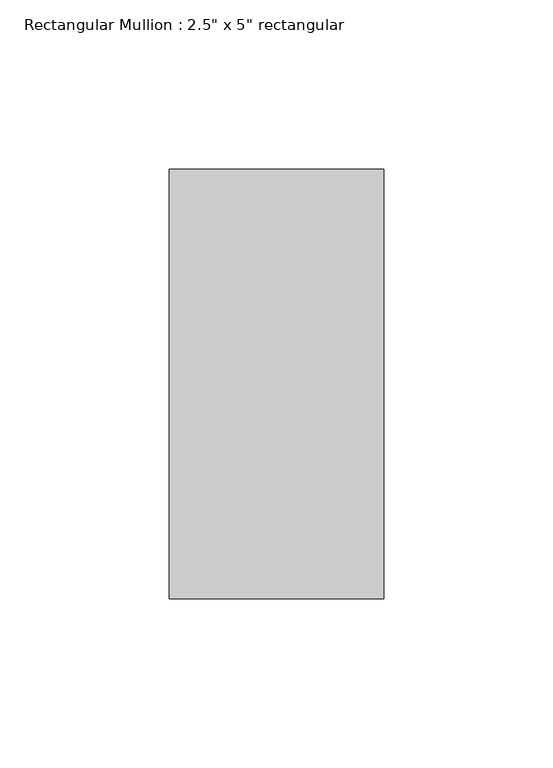
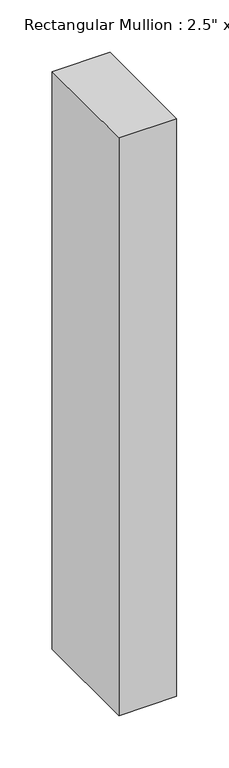
"""IFC4 building model written with IfcOpenShell, lengths in millimetres: member geometry."""

from ifc_helpers import new_model, si_unit, frame, origin, place, context, project, spatial, polyline, outline, extrude, source, transform, mapped, element, save


def member_1e736a25(model_context):
    return source(origin(), model_context, "Body", "SweptSolid", [
        extrude(outline(polyline([(0.0, 63.5), (0.0, -63.5), (-63.5, -63.5), (-63.5, 63.5), (0.0, 63.5)])), frame((0.0, 0.0, -672.1147442), z_axis=(0.0, 0.0, 1.0), x_axis=(1.0, 0.0, 0.0)), (0.0, 0.0, 1.0), 672.1147442),
    ])


if __name__ == "__main__":
    model = new_model("IFC4")
    model_context = context("Model", 3, world=origin())
    ifc_project = project(units=[si_unit("LENGTHUNIT", "METRE", prefix="MILLI")], contexts=[model_context])
    site = spatial("IfcSite", under=ifc_project)
    building = spatial("IfcBuilding", under=site)
    placement = place(None, origin())
    member_shape = member_1e736a25(model_context)
    element("IfcMember", 1, ObjectType="Rectangular Mullion : 2.5\" x 5\" rectangular", at=placement, inside=building, context=model_context, shape_type="MappedRepresentation", body=[
        mapped(member_shape, transform((0.0, 0.0, 0.0), x_axis=(1.0, 0.0, 0.0), y_axis=(0.0, 1.0, 0.0), z_axis=(0.0, 0.0, 1.0))),
    ])
    save(model, "model.ifc")

# Revit data of these elements
# Type "Rectangular Mullion : 2.5\" x 5\" rectangular"
#   built-in parameter 1007304 = 0.416667 (stored number, unit not read)
#   built-in parameter 1007301 = 0.104167 (stored number, unit not read)
#   built-in parameter 1007300 = 0.104167 (stored number, unit not read)
# Element 1 (IfcMember, "Rectangular Mullion : 2.5\" x 5\" rectangular")
#   Materials on its faces: "Aluminum"
# Materials
#   "Aluminum": class "Metal", colour RGB 247 247 247, transparency 0, Description = "Aluminum 6061", Cost = 0
